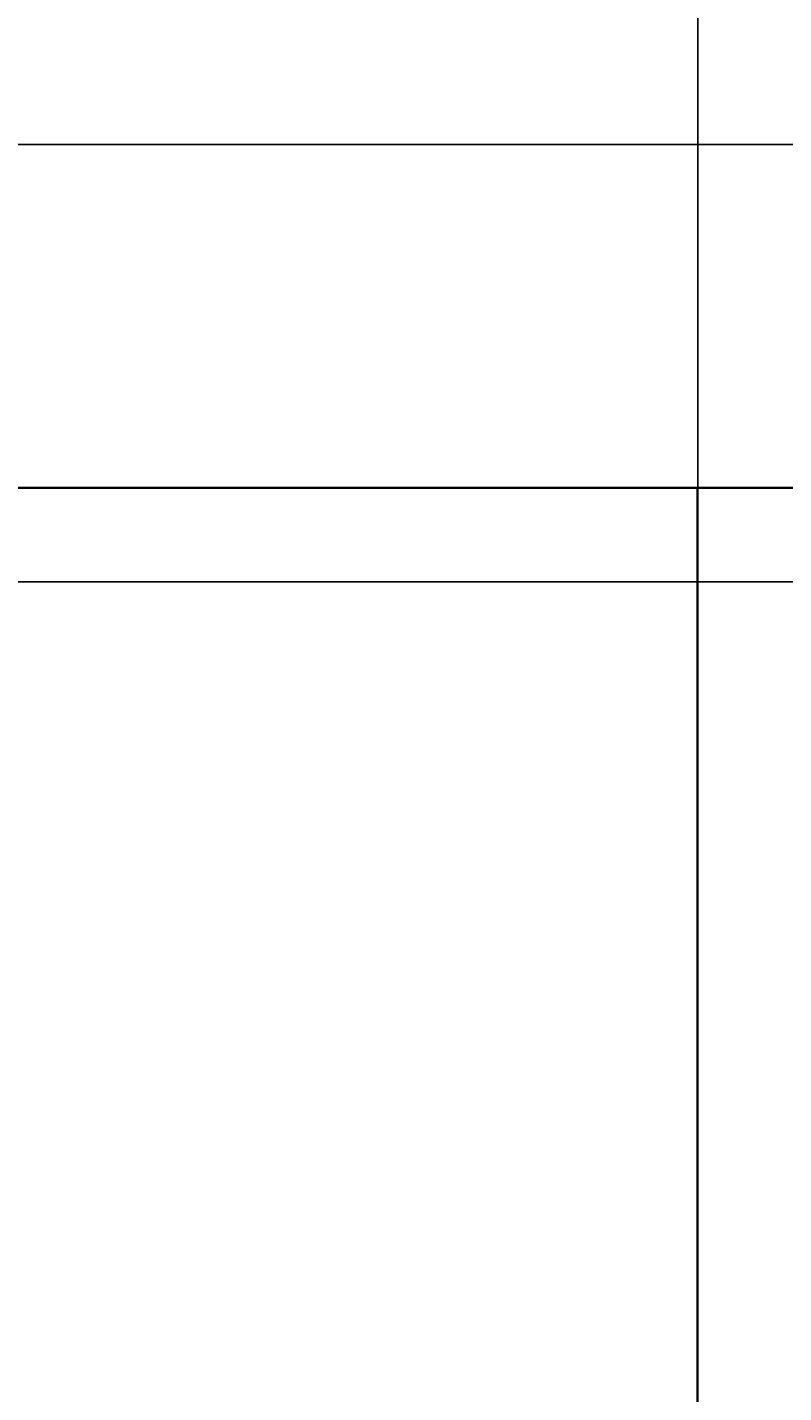
# Model space of a CAD drawing. Units: millimetres. Extents: x 27017497 to 27018854, y 7058029 to 7059154.
# Tile 80 of 91: x 27018246 to 27018319, y 7058503 to 7058634. Entities that reach past the tile are written whole.
import ezdxf

# ---------------------------------------------------------------- set-up
doc = ezdxf.new("R2010")
doc.units = ezdxf.units.MM
doc.layers.add('A-ANNO-DIMS', color=2, linetype='Continuous', lineweight=18)
doc.layers.add('A-WALL', color=7, linetype='Continuous', lineweight=35)
doc.styles.get("Standard").update_dxf_attribs({"font": 'arial.ttf'})
doc.dimstyles.get("Standard").update_dxf_attribs({"dimtxt": 0.18, "dimasz": 0.18, "dimexe": 0.18, "dimexo": 0.0625, "dimgap": 0.09, "dimtad": 0, "dimtih": 1, "dimtoh": 1, "dimdec": 4, "dimzin": 0, "dimdsep": 46, "dimtxsty": 'Standard', "dimcen": 0.09, "dimadec": 0, "dimazin": 0, "dimtfac": 1, "dimtdec": 4, "dimtofl": 0, "dimtmove": 0, "dimatfit": 3, "dimfxl": 1, "dimtolj": 1, "dimtzin": 0, "dimarcsym": 0})

# ---------------------------------------------------------------- blocks, each defined once
blk = doc.blocks.new('*D48')
at = {"layer": 'A-ANNO-DIMS', "color": 0, "lineweight": -2, "transparency": 16777216}
for p, q in [((27018463.5, 7058622.91), (27017497.54, 7058622.91)), ((27017497.72, 7058622.73), (27017497.72, 7058357.75)), ((27017497.72, 7058092.41), (27017497.72, 7058357.39)), ((27018555.13, 7058092.23), (27017497.54, 7058092.23))]:
    blk.add_line(p, q, dxfattribs=at)
at = {"layer": 'A-ANNO-DIMS', "color": 0, "transparency": 16777216}
for points in [[(27017497.69, 7058622.73), (27017497.75, 7058622.73), (27017497.72, 7058622.91)], [(27017497.69, 7058092.41), (27017497.75, 7058092.41), (27017497.72, 7058092.23)]]:
    blk.add_solid(points, dxfattribs=at)
at = {"layer": 'Defpoints', "color": 0, "transparency": 16777216}
for p in [(27018463.56, 7058622.91), (27017497.72, 7058092.23), (27018555.19, 7058092.23)]:
    blk.add_point(p, dxfattribs=at)
at = {"layer": 'A-ANNO-DIMS', "color": 0, "transparency": 16777216, "insert": (27017497.72, 7058357.57), "char_height": 0.18, "attachment_point": 5}
blk.add_mtext('\\A1;530.7', dxfattribs=at)
blk = doc.blocks.new('*D50')
at = {"layer": 'A-ANNO-DIMS', "color": 0, "lineweight": -2, "transparency": 16777216}
for p, q in [((27018223.67, 7058580.91), (27018854.24, 7058580.91)), ((27018854.06, 7058580.73), (27018854.06, 7058511.34)), ((27018854.06, 7058441.59), (27018854.06, 7058510.98)), ((27018223.67, 7058441.41), (27018854.24, 7058441.41))]:
    blk.add_line(p, q, dxfattribs=at)
at = {"layer": 'A-ANNO-DIMS', "color": 0, "transparency": 16777216}
for points in [[(27018854.03, 7058580.73), (27018854.09, 7058580.73), (27018854.06, 7058580.91)], [(27018854.03, 7058441.59), (27018854.09, 7058441.59), (27018854.06, 7058441.41)]]:
    blk.add_solid(points, dxfattribs=at)
at = {"layer": 'Defpoints', "color": 0, "transparency": 16777216}
for p in [(27018223.61, 7058580.91), (27018223.61, 7058441.41), (27018854.06, 7058441.41)]:
    blk.add_point(p, dxfattribs=at)
at = {"layer": 'A-ANNO-DIMS', "color": 0, "transparency": 16777216, "insert": (27018854.06, 7058511.16), "char_height": 0.18, "attachment_point": 5}
blk.add_mtext('\\A1;139.5', dxfattribs=at)
blk = doc.blocks.new('*D52')
at = {"layer": 'A-ANNO-DIMS', "color": 0, "lineweight": -2, "transparency": 16777216}
for p, q in [((27018310.61, 7058589.97), (27018310.61, 7058686.54)), ((27018738.11, 7058589.97), (27018738.11, 7058686.54)), ((27018310.79, 7058686.36), (27018523.96, 7058686.36)), ((27018737.93, 7058686.36), (27018524.75, 7058686.36))]:
    blk.add_line(p, q, dxfattribs=at)
at = {"layer": 'A-ANNO-DIMS', "color": 0, "transparency": 16777216}
for points in [[(27018310.79, 7058686.39), (27018310.79, 7058686.33), (27018310.61, 7058686.36)], [(27018737.93, 7058686.39), (27018737.93, 7058686.33), (27018738.11, 7058686.36)]]:
    blk.add_solid(points, dxfattribs=at)
at = {"layer": 'Defpoints', "color": 0, "transparency": 16777216}
for p in [(27018738.11, 7058686.36), (27018310.61, 7058589.91), (27018738.11, 7058589.91)]:
    blk.add_point(p, dxfattribs=at)
at = {"layer": 'A-ANNO-DIMS', "color": 0, "transparency": 16777216, "insert": (27018524.36, 7058686.36), "char_height": 0.18, "attachment_point": 5}
blk.add_mtext('\\A1;427.5', dxfattribs=at)

msp = doc.modelspace()

# ---------------------------------------------------------------- linework, layer by layer
at = {"layer": 'A-WALL'}
for p, q in [((27017613.666, 7058589.912), (27018310.606, 7058589.912)), ((27018310.606, 7058589.912), (27018310.606, 7058413.839)), ((27018738.106, 7058589.912), (27018310.606, 7058589.912)), ((27018310.606, 7058589.912), (27018310.606, 7058169.223))]:
    msp.add_line(p, q, dxfattribs=at)

# ---------------------------------------------------------------- dimensions: what is measured, and where the dimension line sits
at = {"layer": 'A-ANNO-DIMS'}
dim = msp.add_linear_dim(base=(27018738.106, 7058686.362), p1=(27018310.606, 7058589.912), p2=(27018738.106, 7058589.912), dimstyle='Standard', override={"dimdec": 1, "dimlfac": 1, "dimrnd": 0, "dimzin": 0, "dimdsep": 46, "dimlunit": 2}, dxfattribs=at)
dim.commit()
dim.dimension.update_dxf_attribs({"geometry": '*D52', "text_midpoint": (27018524.356, 7058686.362)})
for base, p1, p2, picture, middle in [((27017497.716, 7058092.23), (27018463.561, 7058622.912), (27018555.192, 7058092.23), '*D48', (27017497.716, 7058357.571)), ((27018854.056, 7058441.412), (27018223.606, 7058580.912), (27018223.606, 7058441.412), '*D50', (27018854.056, 7058511.162))]:
    dim = msp.add_linear_dim(base=base, p1=p1, p2=p2, angle=90, dimstyle='Standard', override={"dimdec": 1, "dimlfac": 1, "dimrnd": 0, "dimzin": 0, "dimdsep": 46, "dimlunit": 2}, dxfattribs=at)
    dim.commit()
    dim.dimension.update_dxf_attribs({"geometry": picture, "text_midpoint": middle})

doc.saveas('drawing.dxf')
